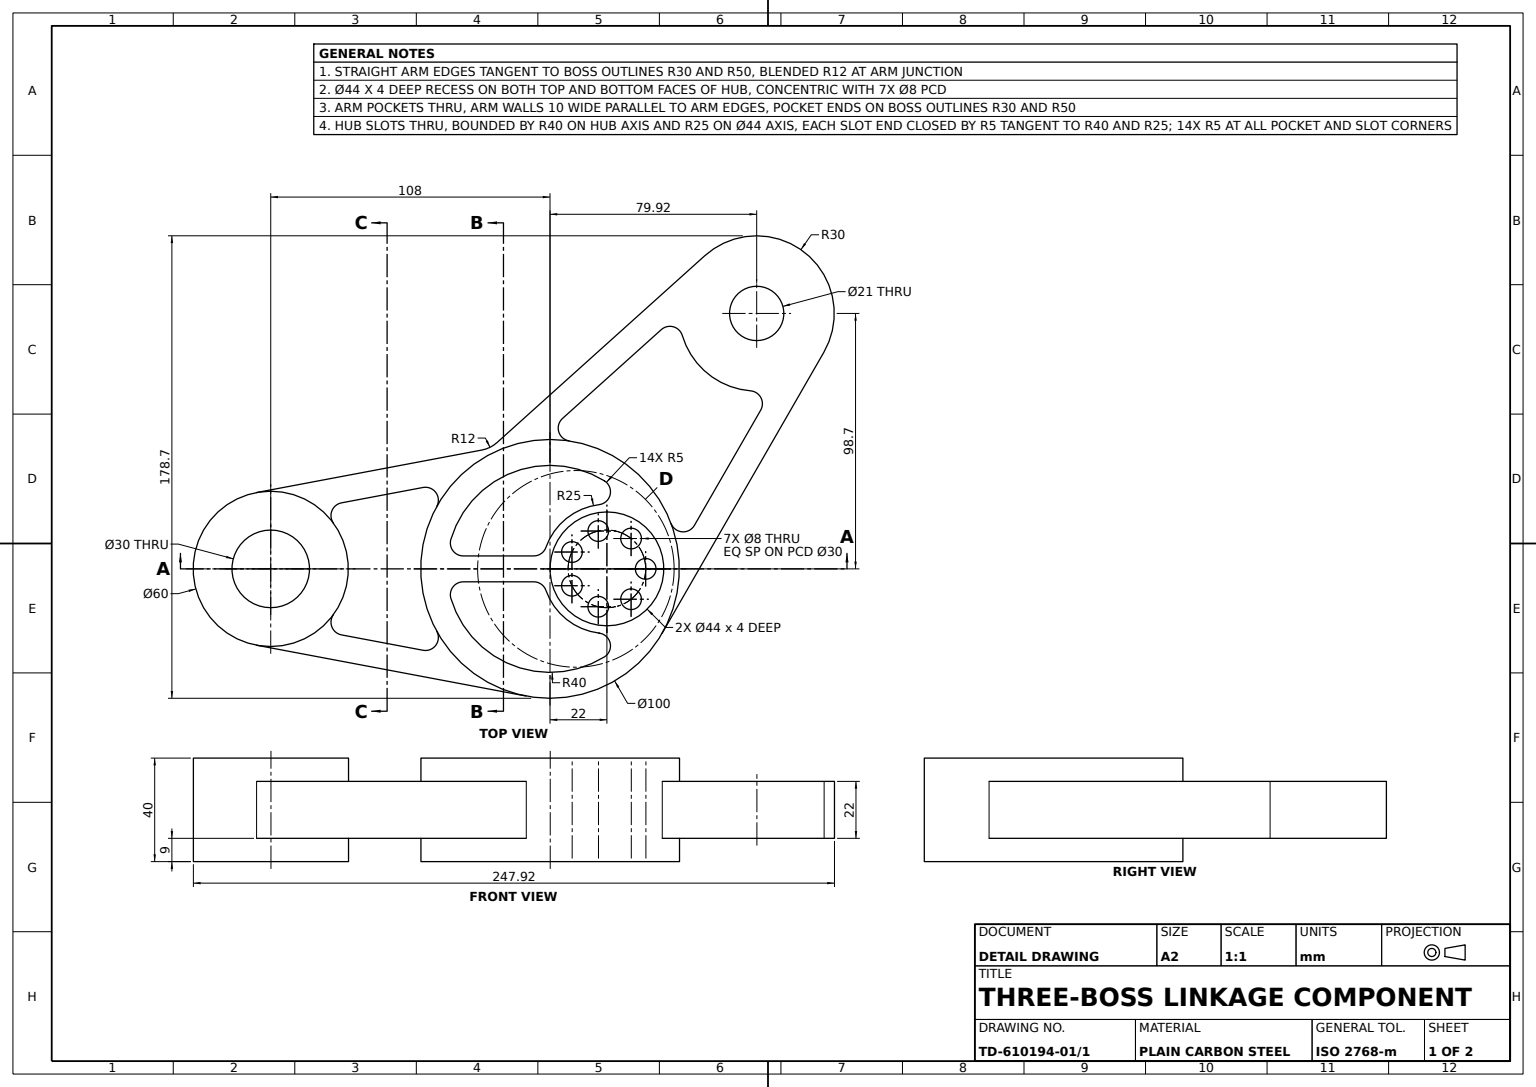
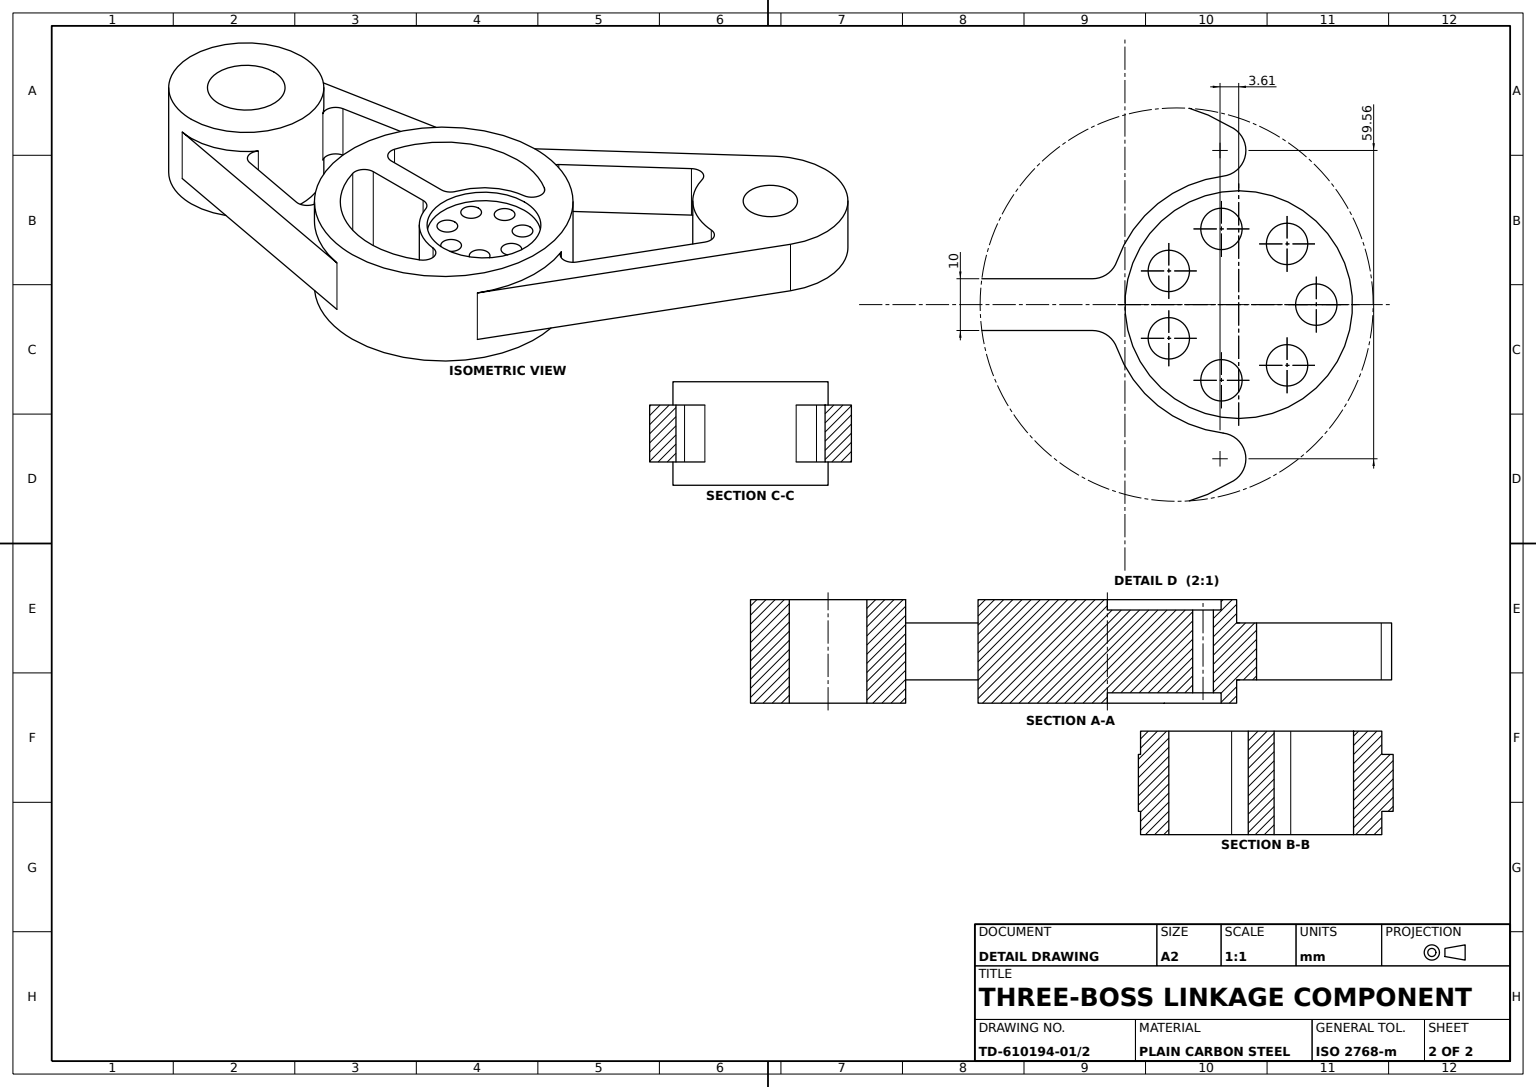
SolidWorks part; units mm, degrees
material "Plain Carbon Steel"
ref_plane "Front Plane" through (0, 0, 0) normal (0, 0, 1) x (1, 0, 0)
ref_plane "Top Plane" through (0, 0, 0) normal (0, 1, 0) x (1, 0, 0)
ref_plane "Right Plane" through (0, 0, 0) normal (1, 0, 0) x (0, 0, -1)
sketch "Hub and Arm Profile Sketch" plane through (0, 0, 0) normal (0, 1, 0) x (1, 0, 0)
  line L0 (-279.5692, 0) -> (340.2253, 0) construction
  line L1 (0, 237.8158) -> (0, -275.9299) construction
  line L2 (-33.541, 5) -> (-6.2843, 5)
  line L3 (-33.541, -5) -> (-6.2843, -5)
  circle A0 centre (0, 0) radius 50
  arc A1 (-38.3326, -11.4286) -> (21.013, -34.0361) centre (0, 0) ccw
  circle A2 centre (-108, 0) radius 30
  arc A4 (-1.5702, -8.3333) -> (18.9886, -24.818) centre (22, 0) ccw
  arc A5 (21.013, 34.0361) -> (-38.3326, 11.4286) centre (0, 0) ccw
  arc A6 (18.9886, 24.818) -> (-1.5702, 8.3333) centre (22, 0) ccw
  arc A7 (-33.541, 5) -> (-38.3326, 11.4286) centre (-33.541, 10) cw
  arc A8 (21.013, -34.0361) -> (18.9886, -24.818) centre (18.3864, -29.7816) ccw
  arc A9 (-6.2843, -5) -> (-1.5702, -8.3333) centre (-6.2843, -10) cw
  arc A10 (21.013, 34.0361) -> (18.9886, 24.818) centre (18.3864, 29.7816) cw
  arc A11 (-1.5702, 8.3333) -> (-6.2843, 5) centre (-6.2843, 10) cw
  arc A12 (-33.541, -5) -> (-38.3326, -11.4286) centre (-33.541, -10) ccw
  circle A13 centre (-108, 0) radius 15
  circle A14 centre (22, 0) radius 15 construction
  circle A15 centre (37, 0) radius 4
  circle A16 centre (31.3523, -11.7275) radius 4
  circle A17 centre (18.6622, -14.6239) radius 4
  circle A18 centre (8.4855, -6.5083) radius 4
  circle A19 centre (8.4855, 6.5083) radius 4
  circle A20 centre (18.6622, 14.6239) radius 4
  circle A21 centre (31.3523, 11.7275) radius 4
  point P25 (33.1591, 22.3713)
  point P49 (22, 0)
  dimension "D1" = 100
  dimension "D2" = 80
  dimension "D3" = 60
  dimension "D5" = 279.5692
  dimension "D7" = 50
  dimension "D9" = 5
  dimension "D10" = 5
  dimension "D11" = 30
  dimension "D12" = 30
  dimension "D13" = 8
  dimension "D4" = 108
  dimension "D6" = 130
  dimension "D8" = 10
  dimension "D15" = 340.2253
  dimension "D16" = 237.8158
  dimension "D17" = 275.9299
  dimension "D18" = 22
  dimension "D14" = 7
extrude "Hub and Arm Body" add sketch "Hub and Arm Profile Sketch" along normal mid plane 40
sketch "Hub Recess Sketch" plane through (0, 20, 0) normal (0, 1, 0) x (1, 0, 0)
  circle A0 centre (22, 0) radius 22
  dimension "D2" = 44
  dimension "D1" = 22
  dimension "D3" = 60.3326
extrude "Hub Recess" cut sketch "Hub Recess Sketch" against normal blind 4
mirror "Hub Recess Mirror" about plane through (0, 0, 0) normal (0, 1, 0) of "Hub Recess"
sketch "Angled Arm Sketch" plane through (0, 0, 0) normal (0, 1, 0) x (1, 0, 0)
  line L0 (-62.0369, 0) -> (95.9548, 0) construction
  line L1 (0, 0) -> (73.4419, 90.6932) construction
  circle A0 centre (79.9237, 98.6975) radius 30
  circle A1 centre (79.9237, 98.6975) radius 10.5
  dimension "D2" = 60
  dimension "D3" = 21
  dimension "D1" = 51
  dimension "D4" = 127
extrude "Angled Arm Boss" add sketch "Angled Arm Sketch" along normal mid plane 22 separate body
sketch "Arm Wall Sketch 1" plane through (0, 0, 0) normal (0, 1, 0) x (1, 0, 0)
  line L0 (-108, 0) -> (58.065, 0) construction
  line L1 (-113.5556, -29.4811) -> (-9.2593, -49.1352)
  line L2 (-80.6279, -25.5101) -> (-49.1, -31.4514)
  line L3 (-113.5556, 29.4811) -> (-9.2593, 49.1352)
  line L4 (-111.7037, -19.6541) -> (-7.4074, -39.3081) construction
  line L5 (-80.6279, 25.5101) -> (-49.1, 31.4514)
  line L6 (-6.2843, -5) -> (-33.541, -5) construction
  line L7 (-33.541, 5) -> (-6.2843, 5) construction
  line L8 (-6.2843, -5) -> (-33.541, -5)
  line L9 (-33.541, 5) -> (-6.2843, 5)
  circle A0 centre (0, 0) radius 50 construction
  circle A1 centre (-108, 0) radius 30 construction
  arc A2 (-43.7946, 24.1254) -> (-43.7946, -24.1254) centre (0, 0) ccw
  arc A3 (-113.5556, 29.4811) -> (-113.5556, -29.4811) centre (-108, 0) ccw
  circle A4 centre (-108, 0) radius 15 construction
  circle A5 centre (-108, 0) radius 15
  circle A6 centre (22, 0) radius 22 construction
  circle A7 centre (22, 0) radius 22
  arc A8 (21.013, 34.0361) -> (-38.3326, 11.4286) centre (0, 0) ccw construction
  arc A9 (21.013, 34.0361) -> (-38.3326, 11.4286) centre (0, 0) ccw
  arc A10 (-38.3326, -11.4286) -> (21.013, -34.0361) centre (0, 0) ccw construction
  arc A11 (21.013, -34.0361) -> (18.9886, -24.818) centre (18.3864, -29.7816) ccw construction
  arc A12 (-33.541, -5) -> (-38.3326, -11.4286) centre (-33.541, -10) ccw construction
  arc A13 (-1.5702, -8.3333) -> (-6.2843, -5) centre (-6.2843, -10) ccw construction
  arc A14 (-1.5702, -8.3333) -> (18.9886, -24.818) centre (22, 0) ccw construction
  arc A15 (-6.2843, 5) -> (-1.5702, 8.3333) centre (-6.2843, 10) ccw construction
  arc A16 (18.9886, 24.818) -> (21.013, 34.0361) centre (18.3864, 29.7816) ccw construction
  arc A17 (18.9886, 24.818) -> (-1.5702, 8.3333) centre (22, 0) ccw construction
  arc A18 (-38.3326, 11.4286) -> (-33.541, 5) centre (-33.541, 10) ccw construction
  arc A19 (-38.3326, -11.4286) -> (21.013, -34.0361) centre (0, 0) ccw
  arc A20 (21.013, -34.0361) -> (18.9886, -24.818) centre (18.3864, -29.7816) ccw
  arc A21 (-33.541, -5) -> (-38.3326, -11.4286) centre (-33.541, -10) ccw
  arc A22 (-1.5702, -8.3333) -> (-6.2843, -5) centre (-6.2843, -10) ccw
  arc A23 (-1.5702, -8.3333) -> (18.9886, -24.818) centre (22, 0) ccw
  arc A24 (-6.2843, 5) -> (-1.5702, 8.3333) centre (-6.2843, 10) ccw
  arc A25 (18.9886, 24.818) -> (21.013, 34.0361) centre (18.3864, 29.7816) ccw
  arc A26 (18.9886, 24.818) -> (-1.5702, 8.3333) centre (22, 0) ccw
  arc A27 (-38.3326, 11.4286) -> (-33.541, 5) centre (-33.541, 10) ccw
  arc A28 (-83.7445, -17.6542) -> (-83.7445, 17.6542) centre (-108, 0) ccw
  arc A29 (-9.2593, -49.1352) -> (-9.2593, 49.1352) centre (0, 0) ccw
  arc A30 (-49.1, 31.4514) -> (-43.7946, 24.1254) centre (-48.1741, 26.5379) cw
  arc A31 (-49.1, -31.4514) -> (-43.7946, -24.1254) centre (-48.1741, -26.5379) ccw
  arc A32 (-80.6279, -25.5101) -> (-83.7445, -17.6542) centre (-79.702, -20.5966) cw
  arc A33 (-80.6279, 25.5101) -> (-83.7445, 17.6542) centre (-79.702, 20.5966) ccw
  point P31 (-36.8885, 33.7526)
  point P41 (-36.8885, -33.7526)
  point P49 (-89.7298, -23.7949)
  point P54 (-89.7298, 23.7949)
  dimension "D2" = 5
  dimension "D1" = 10
extrude "Arm Wall Boss 1" add sketch "Arm Wall Sketch 1" along normal mid plane 22
sketch "Arm Wall Sketch 2" plane through (0, 0, 0) normal (0, 1, 0) x (1, 0, 0)
  line L0 (-49.1, 31.4514) -> (-80.6279, 25.5101) construction
  line L1 (-9.2593, 49.1352) -> (-113.5556, 29.4811) construction
  line L2 (-49.1, 31.4514) -> (-80.6279, 25.5101)
  line L3 (-26.3092, 45.9222) -> (-113.5556, 29.4811)
  line L4 (0, 0) -> (79.9237, 98.6975) construction
  line L5 (43.3277, -24.9541) -> (105.9203, 83.7251)
  line L6 (55.8365, 16.8015) -> (81.4724, 61.313)
  line L7 (-20.5113, 48.7884) -> (59.8734, 121.0131)
  line L8 (34.6622, -19.9633) -> (97.2548, 88.7159) construction
  line L9 (4.8253, 58.1095) -> (43.0341, 92.4397)
  line L11 (-33.541, 5) -> (-6.2843, 5)
  line L12 (-33.541, 5) -> (-6.2843, 5)
  line L13 (-6.2843, -5) -> (-33.541, -5)
  line L14 (-6.2843, -5) -> (-33.541, -5)
  arc A0 (-43.7946, 24.1254) -> (-49.1, 31.4514) centre (-48.1741, 26.5379) ccw construction
  arc A1 (-80.6279, 25.5101) -> (-83.7445, 17.6542) centre (-79.702, 20.5966) ccw construction
  arc A2 (-83.7445, 17.6542) -> (-113.5556, 29.4811) centre (-108, 0) ccw construction
  circle A3 centre (0, 0) radius 50 construction
  circle A4 centre (79.9237, 98.6975) radius 30 construction
  circle A5 centre (79.9237, 98.6975) radius 10.5 construction
  arc A6 (-43.7946, 24.1254) -> (-49.1, 31.4514) centre (-48.1741, 26.5379) ccw
  arc A7 (-80.6279, 25.5101) -> (-83.7445, 17.6542) centre (-79.702, 20.5966) ccw
  arc A8 (-83.7445, 17.6542) -> (-113.5556, 29.4811) centre (-108, 0) ccw
  arc A9 (46.8215, 17.5426) -> (7.4245, 49.4457) centre (0, 0) ccw
  arc A10 (105.9203, 83.7251) -> (59.8734, 121.0131) centre (79.9237, 98.6975) ccw
  circle A11 centre (79.9237, 98.6975) radius 10.5
  arc A12 (55.8365, 16.8015) -> (46.8215, 17.5426) centre (51.5037, 19.2969) cw
  arc A13 (81.4724, 61.313) -> (77.5374, 68.7926) centre (77.1396, 63.8084) ccw
  arc A14 (4.8253, 58.1095) -> (7.4245, 49.4457) centre (8.167, 54.3903) ccw
  arc A15 (43.0341, 92.4397) -> (51.1684, 90.1458) centre (46.3758, 88.7205) cw
  arc A16 (-20.5113, 48.7884) -> (-26.3092, 45.9222) centre (-28.5314, 57.7147) cw
  arc A17 (-43.7946, 24.1254) -> (43.3277, -24.9541) centre (0, 0) ccw
  circle A18 centre (22, 0) radius 22 construction
  circle A19 centre (22, 0) radius 22
  arc A20 (51.1684, 90.1458) -> (77.5374, 68.7926) centre (79.9237, 98.6975) ccw
  arc A23 (-38.3326, 11.4286) -> (-33.541, 5) centre (-33.541, 10) ccw
  arc A24 (21.013, 34.0361) -> (-38.3326, 11.4286) centre (0, 0) ccw
  arc A25 (18.9886, 24.818) -> (21.013, 34.0361) centre (18.3864, 29.7816) ccw
  arc A26 (18.9886, 24.818) -> (-1.5702, 8.3333) centre (22, 0) ccw
  arc A27 (-6.2843, 5) -> (-1.5702, 8.3333) centre (-6.2843, 10) ccw
  arc A28 (-38.3326, 11.4286) -> (-33.541, 5) centre (-33.541, 10) ccw
  arc A29 (21.013, 34.0361) -> (-38.3326, 11.4286) centre (0, 0) ccw
  arc A30 (18.9886, 24.818) -> (21.013, 34.0361) centre (18.3864, 29.7816) ccw
  arc A31 (18.9886, 24.818) -> (-1.5702, 8.3333) centre (22, 0) ccw
  arc A32 (-6.2843, 5) -> (-1.5702, 8.3333) centre (-6.2843, 10) ccw
  arc A33 (-1.5702, -8.3333) -> (18.9886, -24.818) centre (22, 0) ccw
  arc A34 (21.013, -34.0361) -> (18.9886, -24.818) centre (18.3864, -29.7816) ccw
  arc A35 (-38.3326, -11.4286) -> (21.013, -34.0361) centre (0, 0) ccw
  arc A36 (-33.541, -5) -> (-38.3326, -11.4286) centre (-33.541, -10) ccw
  arc A37 (-1.5702, -8.3333) -> (-6.2843, -5) centre (-6.2843, -10) ccw
  arc A38 (-1.5702, -8.3333) -> (18.9886, -24.818) centre (22, 0) ccw
  arc A39 (21.013, -34.0361) -> (18.9886, -24.818) centre (18.3864, -29.7816) ccw
  arc A40 (-38.3326, -11.4286) -> (21.013, -34.0361) centre (0, 0) ccw
  arc A41 (-33.541, -5) -> (-38.3326, -11.4286) centre (-33.541, -10) ccw
  arc A42 (-1.5702, -8.3333) -> (-6.2843, -5) centre (-6.2843, -10) ccw
  dimension "D2" = 5
  dimension "D3" = 5
  dimension "D4" = 12
  dimension "D1" = 10
  dimension "D5" = 0
  dimension "D6" = 0
extrude "Arm Wall Boss 2" add sketch "Arm Wall Sketch 2" along normal mid plane 22
